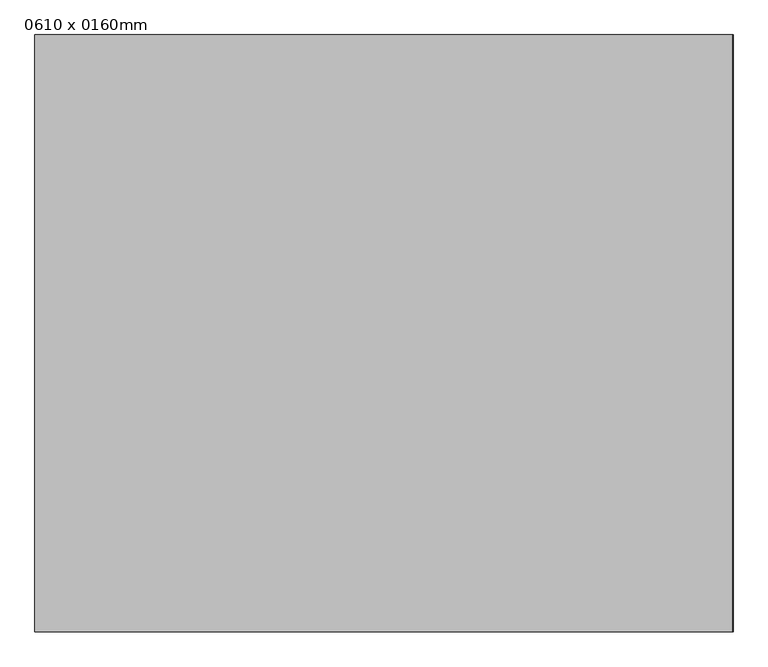
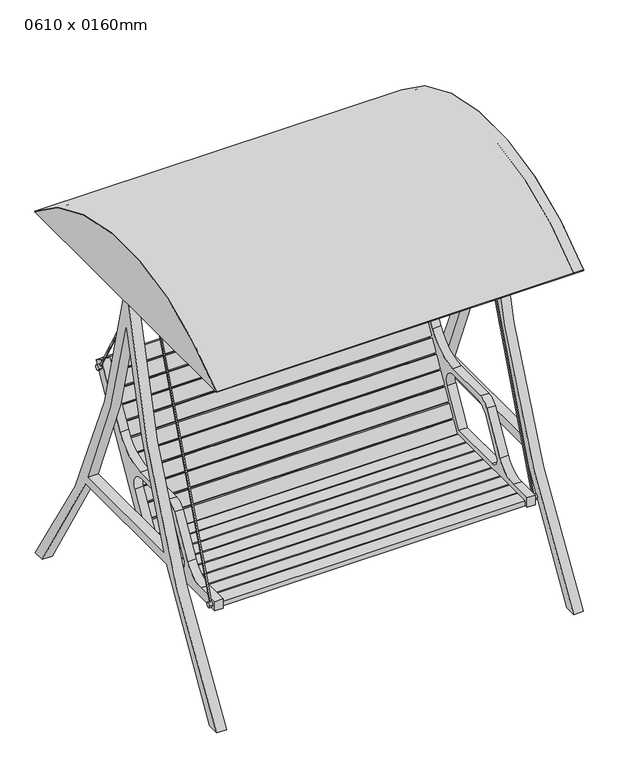
"""IFC4 building model written with IfcOpenShell, lengths in millimetres: furniture geometry, 0610 x 0160mm."""

from ifc_helpers import new_model, si_unit, point, frame, frame_2d, origin, place, context, project, spatial, polyline, circle_curve, trimmed, segment, composite_curve, outline, extrude, source, transform, mapped, element, save


def furniture_0610_x_0160mm_a8fad5e2(model_context):
    return source(origin(), model_context, "Body", "SweptSolid", [
        extrude(outline(composite_curve([segment(trimmed(circle_curve(frame_2d((4189.9023331, 1950.2809332)), 3303.1244251), [point((933.45, 1396.9734505))], [point((1524.0, 0.0))], True, "CARTESIAN"), True, "CONTINUOUS"), segment(polyline([(1524.0, 0.0), (1476.936255, 0.0)]), True, "CONTINUOUS"), segment(trimmed(circle_curve(frame_2d((4189.9023331, 1950.2809332)), 3341.2244251), [point((1476.936255, 0.0))], [point((1186.3373595, 486.5944542))], False, "CARTESIAN"), True, "CONTINUOUS"), segment(polyline([(1186.3373595, 486.5944542), (642.4626405, 486.5944542)]), True, "CONTINUOUS"), segment(trimmed(circle_curve(frame_2d((-2361.1023331, 1950.2809332)), 3341.2244251), [point((642.4626405, 486.5944542))], [point((351.863745, 0.0))], False, "CARTESIAN"), True, "CONTINUOUS"), segment(polyline([(351.863745, 0.0), (304.8, 0.0)]), True, "CONTINUOUS"), segment(trimmed(circle_curve(frame_2d((-2361.1023331, 1950.2809332)), 3303.1244251), [point((304.8, 0.0))], [point((895.35, 1396.9734505))], True, "CARTESIAN"), True, "CONTINUOUS"), segment(polyline([(895.35, 1396.9734505), (895.35, 1524.0), (914.4, 1524.0), (933.45, 1524.0), (933.45, 1396.9734505)]), True, "CONTINUOUS")], self_intersect=False), holes=[composite_curve([segment(polyline([(660.7321842, 524.6944542), (1168.0678158, 524.6944542)]), True, "CONTINUOUS"), segment(trimmed(circle_curve(frame_2d((4189.9023331, 1950.2809332)), 3341.2244251), [point((1168.0678158, 524.6944542))], [point((914.4, 1290.8378915))], False, "CARTESIAN"), True, "CONTINUOUS"), segment(trimmed(circle_curve(frame_2d((-2361.1023331, 1950.2809332)), 3341.2244251), [point((914.4, 1290.8378915))], [point((660.7321842, 524.6944542))], False, "CARTESIAN"), True, "CONTINUOUS")], self_intersect=False)]), frame((-272.362745, 0.0, 0.0), z_axis=(1.0, 0.0, 0.0), x_axis=(0.0, 1.0, 0.0)), (0.0, 0.0, 1.0), 38.1),
        extrude(outline(composite_curve([segment(trimmed(circle_curve(frame_2d((4189.9023331, 1950.2809332)), 3303.1244251), [point((933.45, 1396.9734505))], [point((1524.0, 0.0))], True, "CARTESIAN"), True, "CONTINUOUS"), segment(polyline([(1524.0, 0.0), (1476.936255, 0.0)]), True, "CONTINUOUS"), segment(trimmed(circle_curve(frame_2d((4189.9023331, 1950.2809332)), 3341.2244251), [point((1476.936255, 0.0))], [point((1186.3373595, 486.5944542))], False, "CARTESIAN"), True, "CONTINUOUS"), segment(polyline([(1186.3373595, 486.5944542), (642.4626405, 486.5944542)]), True, "CONTINUOUS"), segment(trimmed(circle_curve(frame_2d((-2361.1023331, 1950.2809332)), 3341.2244251), [point((642.4626405, 486.5944542))], [point((351.863745, 0.0))], False, "CARTESIAN"), True, "CONTINUOUS"), segment(polyline([(351.863745, 0.0), (304.8, 0.0)]), True, "CONTINUOUS"), segment(trimmed(circle_curve(frame_2d((-2361.1023331, 1950.2809332)), 3303.1244251), [point((304.8, 0.0))], [point((895.35, 1396.9734505))], True, "CARTESIAN"), True, "CONTINUOUS"), segment(polyline([(895.35, 1396.9734505), (895.35, 1524.0), (914.4, 1524.0), (933.45, 1524.0), (933.45, 1396.9734505)]), True, "CONTINUOUS")], self_intersect=False), holes=[composite_curve([segment(polyline([(660.7321842, 524.6944542), (1168.0678158, 524.6944542)]), True, "CONTINUOUS"), segment(trimmed(circle_curve(frame_2d((4189.9023331, 1950.2809332)), 3341.2244251), [point((1168.0678158, 524.6944542))], [point((914.4, 1290.8378915))], False, "CARTESIAN"), True, "CONTINUOUS"), segment(trimmed(circle_curve(frame_2d((-2361.1023331, 1950.2809332)), 3341.2244251), [point((914.4, 1290.8378915))], [point((660.7321842, 524.6944542))], False, "CARTESIAN"), True, "CONTINUOUS")], self_intersect=False)]), frame((1111.937255, 0.0, 0.0), z_axis=(1.0, 0.0, 0.0), x_axis=(0.0, 1.0, 0.0)), (0.0, 0.0, 1.0), 38.1),
        extrude(outline(polyline([(1111.937255, 933.45), (1111.937255, 895.35), (-234.262745, 895.35), (-234.262745, 933.45), (1111.937255, 933.45)])), frame((0.0, 0.0, 1484.1023899), z_axis=(0.0, 0.0, 1.0), x_axis=(1.0, 0.0, 0.0)), (0.0, 0.0, 1.0), 39.8976101),
        extrude(outline(composite_curve([segment(trimmed(circle_curve(frame_2d((914.4, 699.3747703)), 926.421113), [point((304.8, 1396.9734505))], [point((1524.0, 1396.9734505))], False, "CARTESIAN"), True, "CONTINUOUS"), segment(polyline([(1524.0, 1396.9734505), (304.8, 1396.9734505)]), True, "CONTINUOUS")], self_intersect=False), holes=[composite_curve([segment(polyline([(376.708681, 1422.3734505), (1452.091319, 1422.3734505)]), True, "CONTINUOUS"), segment(trimmed(circle_curve(frame_2d((914.4, 699.3747703)), 901.021113), [point((1452.091319, 1422.3734505))], [point((376.708681, 1422.3734505))], True, "CARTESIAN"), True, "CONTINUOUS")], self_intersect=False)]), frame((-272.362745, 0.0, 0.0), z_axis=(1.0, 0.0, 0.0), x_axis=(0.0, 1.0, 0.0)), (0.0, 0.0, 1.0), 38.1),
        extrude(outline(composite_curve([segment(trimmed(circle_curve(frame_2d((914.4, 699.3747703)), 926.421113), [point((304.8, 1396.9734505))], [point((1524.0, 1396.9734505))], False, "CARTESIAN"), True, "CONTINUOUS"), segment(polyline([(1524.0, 1396.9734505), (304.8, 1396.9734505)]), True, "CONTINUOUS")], self_intersect=False), holes=[composite_curve([segment(polyline([(376.708681, 1422.3734505), (1452.091319, 1422.3734505)]), True, "CONTINUOUS"), segment(trimmed(circle_curve(frame_2d((914.4, 699.3747703)), 901.021113), [point((1452.091319, 1422.3734505))], [point((376.708681, 1422.3734505))], True, "CARTESIAN"), True, "CONTINUOUS")], self_intersect=False)]), frame((1111.937255, 0.0, 0.0), z_axis=(1.0, 0.0, 0.0), x_axis=(0.0, 1.0, 0.0)), (0.0, 0.0, 1.0), 38.1),
        extrude(outline(composite_curve([segment(trimmed(circle_curve(frame_2d((914.4, 699.3747703)), 926.421113), [point((304.8, 1396.9734505))], [point((1524.0, 1396.9734505))], False, "CARTESIAN"), True, "CONTINUOUS"), segment(polyline([(1524.0, 1396.9734505), (304.8, 1396.9734505)]), True, "CONTINUOUS")], self_intersect=False)), frame((-273.952745, 0.0, 0.0), z_axis=(1.0, 0.0, 0.0), x_axis=(0.0, 1.0, 0.0)), (0.0, 0.0, 1.0), 1.59),
        extrude(outline(composite_curve([segment(trimmed(circle_curve(frame_2d((914.4, 699.3747703)), 926.421113), [point((304.8, 1396.9734505))], [point((1524.0, 1396.9734505))], False, "CARTESIAN"), True, "CONTINUOUS"), segment(polyline([(1524.0, 1396.9734505), (304.8, 1396.9734505)]), True, "CONTINUOUS")], self_intersect=False)), frame((1150.037255, 0.0, 0.0), z_axis=(1.0, 0.0, 0.0), x_axis=(0.0, 1.0, 0.0)), (0.0, 0.0, 1.0), 1.59),
        extrude(outline(composite_curve([segment(trimmed(circle_curve(frame_2d((914.4, 699.3747703)), 926.421113), [point((1524.0, 1396.9734505))], [point((304.8, 1396.9734505))], True, "CARTESIAN"), True, "CONTINUOUS"), segment(polyline([(304.8, 1396.9734505), (304.8, 1399.0836139)]), True, "CONTINUOUS"), segment(trimmed(circle_curve(frame_2d((914.4, 699.3747703)), 928.011113), [point((304.8, 1399.0836139))], [point((1524.0, 1399.0836139))], False, "CARTESIAN"), True, "CONTINUOUS"), segment(polyline([(1524.0, 1399.0836139), (1524.0, 1396.9734505)]), True, "CONTINUOUS")], self_intersect=False)), frame((-273.952745, 0.0, 0.0), z_axis=(1.0, 0.0, 0.0), x_axis=(0.0, 1.0, 0.0)), (0.0, 0.0, 1.0), 1423.99),
        extrude(outline(composite_curve([segment(trimmed(circle_curve(frame_2d((563.6419667, 511.4)), 105.0), [point((563.6419667, 406.4))], [point((654.5746341, 458.9))], True, "CARTESIAN"), True, "CONTINUOUS"), segment(polyline([(654.5746341, 458.9), (741.8122598, 610.0)]), True, "CONTINUOUS"), segment(trimmed(circle_curve(frame_2d((785.11353, 585.0)), 50.0), [point((741.8122598, 610.0))], [point((785.11353, 635.0))], False, "CARTESIAN"), True, "CONTINUOUS"), segment(polyline([(785.11353, 635.0), (968.6699734, 635.0)]), True, "CONTINUOUS"), segment(trimmed(circle_curve(frame_2d((968.6699734, 795.0)), 160.0), [point((968.6699734, 635.0))], [point((1107.2340381, 715.0))], True, "CARTESIAN"), True, "CONTINUOUS"), segment(polyline([(1107.2340381, 715.0), (1233.863745, 934.3290861), (1266.8593129, 915.2790861), (951.0607902, 368.3), (471.863745, 368.3), (471.863745, 406.4), (563.6419667, 406.4)]), True, "CONTINUOUS")], self_intersect=False), holes=[composite_curve([segment(trimmed(circle_curve(frame_2d((807.1413638, 546.8466726)), 62.7533274), [point((807.1413638, 609.6))], [point((752.7953881, 578.2233363))], True, "CARTESIAN"), True, "CONTINUOUS"), segment(polyline([(752.7953881, 578.2233363), (679.5739008, 451.4)]), True, "CONTINUOUS"), segment(trimmed(circle_curve(frame_2d((705.5546629, 436.4)), 30.0), [point((679.5739008, 451.4))], [point((705.5546629, 406.4))], True, "CARTESIAN"), True, "CONTINUOUS"), segment(polyline([(705.5546629, 406.4), (929.063745, 406.4), (1007.4101765, 542.1)]), True, "CONTINUOUS"), segment(trimmed(circle_curve(frame_2d((968.4390333, 564.6)), 45.0), [point((1007.4101765, 542.1))], [point((968.4390333, 609.6))], True, "CARTESIAN"), True, "CONTINUOUS"), segment(polyline([(968.4390333, 609.6), (807.1413638, 609.6)]), True, "CONTINUOUS")], self_intersect=False)]), frame((-184.03019, 0.0, 0.0), z_axis=(1.0, 0.0, 0.0), x_axis=(0.0, 1.0, 0.0)), (0.0, 0.0, 1.0), 32.5713093),
        extrude(outline(composite_curve([segment(trimmed(circle_curve(frame_2d((563.6419667, 511.4)), 105.0), [point((563.6419667, 406.4))], [point((654.5746341, 458.9))], True, "CARTESIAN"), True, "CONTINUOUS"), segment(polyline([(654.5746341, 458.9), (741.8122598, 610.0)]), True, "CONTINUOUS"), segment(trimmed(circle_curve(frame_2d((785.11353, 585.0)), 50.0), [point((741.8122598, 610.0))], [point((785.11353, 635.0))], False, "CARTESIAN"), True, "CONTINUOUS"), segment(polyline([(785.11353, 635.0), (968.6699734, 635.0)]), True, "CONTINUOUS"), segment(trimmed(circle_curve(frame_2d((968.6699734, 795.0)), 160.0), [point((968.6699734, 635.0))], [point((1107.2340381, 715.0))], True, "CARTESIAN"), True, "CONTINUOUS"), segment(polyline([(1107.2340381, 715.0), (1233.863745, 934.3290861), (1266.8593129, 915.2790861), (951.0607902, 368.3), (471.863745, 368.3), (471.863745, 406.4), (563.6419667, 406.4)]), True, "CONTINUOUS")], self_intersect=False), holes=[composite_curve([segment(trimmed(circle_curve(frame_2d((807.1413638, 546.8466726)), 62.7533274), [point((807.1413638, 609.6))], [point((752.7953881, 578.2233363))], True, "CARTESIAN"), True, "CONTINUOUS"), segment(polyline([(752.7953881, 578.2233363), (679.5739008, 451.4)]), True, "CONTINUOUS"), segment(trimmed(circle_curve(frame_2d((705.5546629, 436.4)), 30.0), [point((679.5739008, 451.4))], [point((705.5546629, 406.4))], True, "CARTESIAN"), True, "CONTINUOUS"), segment(polyline([(705.5546629, 406.4), (929.063745, 406.4), (1007.4101765, 542.1)]), True, "CONTINUOUS"), segment(trimmed(circle_curve(frame_2d((968.4390333, 564.6)), 45.0), [point((1007.4101765, 542.1))], [point((968.4390333, 609.6))], True, "CARTESIAN"), True, "CONTINUOUS"), segment(polyline([(968.4390333, 609.6), (807.1413638, 609.6)]), True, "CONTINUOUS")], self_intersect=False)]), frame((1027.5433908, 0.0, 0.0), z_axis=(1.0, 0.0, 0.0), x_axis=(0.0, 1.0, 0.0)), (0.0, 0.0, 1.0), 32.5713093),
        extrude(outline(polyline([(0.0, -19.0500001), (0.0, 0.0), (1179.0022715, 0.0), (1179.0022715, -19.0500001), (0.0, -19.0500001)])), frame((1027.5433908, 1224.9615289, 880.8099956), z_axis=(0.0, 0.5000000000000067, 0.8660254037844349), x_axis=(-1.0, 0.0, 0.0)), (0.0, 0.0, 1.0), 50.8),
        extrude(outline(polyline([(0.0, -19.0500001), (0.0, 0.0), (1179.0022715, 0.0), (1179.0022715, -19.0500001), (0.0, -19.0500001)])), frame((1027.5433908, 1196.3865289, 831.3166438), z_axis=(0.0, 0.5000000000000067, 0.8660254037844349), x_axis=(-1.0, 0.0, 0.0)), (0.0, 0.0, 1.0), 50.8),
        extrude(outline(polyline([(0.0, -19.0500001), (0.0, 0.0), (1179.0022715, 0.0), (1179.0022715, -19.0500001), (0.0, -19.0500001)])), frame((1027.5433908, 1167.8115289, 781.823292), z_axis=(0.0, 0.5000000000000067, 0.8660254037844349), x_axis=(-1.0, 0.0, 0.0)), (0.0, 0.0, 1.0), 50.8),
        extrude(outline(polyline([(0.0, -19.0500001), (0.0, 0.0), (1179.0022715, 0.0), (1179.0022715, -19.0500001), (0.0, -19.0500001)])), frame((1027.5433908, 1139.2365289, 732.3299402), z_axis=(0.0, 0.5000000000000067, 0.8660254037844349), x_axis=(-1.0, 0.0, 0.0)), (0.0, 0.0, 1.0), 50.8),
        extrude(outline(polyline([(0.0, -19.0500001), (0.0, 0.0), (1179.0022715, 0.0), (1179.0022715, -19.0500001), (0.0, -19.0500001)])), frame((1027.5433908, 1110.6615289, 682.8365883), z_axis=(0.0, 0.5000000000000067, 0.8660254037844349), x_axis=(-1.0, 0.0, 0.0)), (0.0, 0.0, 1.0), 50.8),
        extrude(outline(polyline([(0.0, -19.0500001), (0.0, 0.0), (1179.0022715, 0.0), (1179.0022715, -19.0500001), (0.0, -19.0500001)])), frame((1027.5433908, 1082.0865289, 633.3432365), z_axis=(0.0, 0.5000000000000067, 0.8660254037844349), x_axis=(-1.0, 0.0, 0.0)), (0.0, 0.0, 1.0), 50.8),
        extrude(outline(polyline([(0.0, -19.0500001), (0.0, 0.0), (1179.0022715, 0.0), (1179.0022715, -19.0500001), (0.0, -19.0500001)])), frame((1027.5433908, 1053.5115289, 583.8498847), z_axis=(0.0, 0.5000000000000067, 0.8660254037844349), x_axis=(-1.0, 0.0, 0.0)), (0.0, 0.0, 1.0), 50.8),
        extrude(outline(polyline([(0.0, -19.0500001), (0.0, 0.0), (1179.0022715, 0.0), (1179.0022715, -19.0500001), (0.0, -19.0500001)])), frame((1027.5433908, 1024.9365289, 534.3565329), z_axis=(0.0, 0.5000000000000067, 0.8660254037844349), x_axis=(-1.0, 0.0, 0.0)), (0.0, 0.0, 1.0), 50.8),
        extrude(outline(polyline([(0.0, -19.0500001), (0.0, 0.0), (1179.0022715, 0.0), (1179.0022715, -19.0500001), (0.0, -19.0500001)])), frame((1027.5433908, 996.3615289, 484.863181), z_axis=(0.0, 0.5000000000000067, 0.8660254037844349), x_axis=(-1.0, 0.0, 0.0)), (0.0, 0.0, 1.0), 50.8),
        extrude(outline(polyline([(0.0, -19.0500001), (0.0, 0.0), (1179.0022715, 0.0), (1179.0022715, -19.0500001), (0.0, -19.0500001)])), frame((1027.5433908, 967.7865289, 435.3698292), z_axis=(0.0, 0.5000000000000067, 0.8660254037844349), x_axis=(-1.0, 0.0, 0.0)), (0.0, 0.0, 1.0), 50.8),
        extrude(outline(polyline([(0.0, -19.0500001), (0.0, 0.0), (1179.0022715, 0.0), (1179.0022715, -19.0500001), (0.0, -19.0500001)])), frame((1027.5433908, 939.2115289, 385.8764774), z_axis=(0.0, 0.5000000000000067, 0.8660254037844349), x_axis=(-1.0, 0.0, 0.0)), (0.0, 0.0, 1.0), 50.8),
        extrude(outline(polyline([(1027.5433908, 933.8211), (1027.5433908, 883.0211), (-151.4588807, 883.0211), (-151.4588807, 933.8211), (1027.5433908, 933.8211)])), frame((0.0, 0.0, 368.3), z_axis=(0.0, 0.0, 1.0), x_axis=(1.0, 0.0, 0.0)), (0.0, 0.0, 1.0), 19.05),
        extrude(outline(polyline([(1027.5433908, 876.6711), (1027.5433908, 825.8711), (-151.4588807, 825.8711), (-151.4588807, 876.6711), (1027.5433908, 876.6711)])), frame((0.0, 0.0, 368.3), z_axis=(0.0, 0.0, 1.0), x_axis=(1.0, 0.0, 0.0)), (0.0, 0.0, 1.0), 19.05),
        extrude(outline(polyline([(1027.5433908, 819.5211), (1027.5433908, 768.7211), (-151.4588807, 768.7211), (-151.4588807, 819.5211), (1027.5433908, 819.5211)])), frame((0.0, 0.0, 368.3), z_axis=(0.0, 0.0, 1.0), x_axis=(1.0, 0.0, 0.0)), (0.0, 0.0, 1.0), 19.05),
        extrude(outline(polyline([(1027.5433908, 762.3711), (1027.5433908, 711.5711), (-151.4588807, 711.5711), (-151.4588807, 762.3711), (1027.5433908, 762.3711)])), frame((0.0, 0.0, 368.3), z_axis=(0.0, 0.0, 1.0), x_axis=(1.0, 0.0, 0.0)), (0.0, 0.0, 1.0), 19.05),
        extrude(outline(polyline([(1027.5433908, 705.2211), (1027.5433908, 654.4211), (-151.4588807, 654.4211), (-151.4588807, 705.2211), (1027.5433908, 705.2211)])), frame((0.0, 0.0, 368.3), z_axis=(0.0, 0.0, 1.0), x_axis=(1.0, 0.0, 0.0)), (0.0, 0.0, 1.0), 19.05),
        extrude(outline(polyline([(1027.5433908, 648.0711), (1027.5433908, 597.2711), (-151.4588807, 597.2711), (-151.4588807, 648.0711), (1027.5433908, 648.0711)])), frame((0.0, 0.0, 368.3), z_axis=(0.0, 0.0, 1.0), x_axis=(1.0, 0.0, 0.0)), (0.0, 0.0, 1.0), 19.05),
        extrude(outline(polyline([(1027.5433908, 590.9211), (1027.5433908, 540.1211), (-151.4588807, 540.1211), (-151.4588807, 590.9211), (1027.5433908, 590.9211)])), frame((0.0, 0.0, 368.3), z_axis=(0.0, 0.0, 1.0), x_axis=(1.0, 0.0, 0.0)), (0.0, 0.0, 1.0), 19.05),
        extrude(outline(polyline([(1027.5433908, 533.7711), (1027.5433908, 482.9711), (-151.4588807, 482.9711), (-151.4588807, 533.7711), (1027.5433908, 533.7711)])), frame((0.0, 0.0, 368.3), z_axis=(0.0, 0.0, 1.0), x_axis=(1.0, 0.0, 0.0)), (0.0, 0.0, 1.0), 19.05),
        extrude(outline(polyline([(914.4, 1484.1023899), (1241.1891484, 905.4891111), (1236.3748088, 902.7700689), (911.842017, 1477.3882398), (494.9813942, 383.2195737), (489.4362629, 385.3321793), (908.05, 1484.1023899), (914.4, 1484.1023899)])), frame((-188.7825876, 0.0, 0.0), z_axis=(1.0, 0.0, 0.0), x_axis=(0.0, 1.0, 0.0)), (0.0, 0.0, 1.0), 4.7523976),
        extrude(outline(composite_curve([segment(trimmed(circle_curve(frame_2d((1238.7819786, 904.12959)), 10.0), [point((1228.7819786, 904.12959))], [point((1248.7819786, 904.12959))], False, "CARTESIAN"), True, "CONTINUOUS"), segment(trimmed(circle_curve(frame_2d((1238.7819786, 904.12959)), 10.0), [point((1248.7819786, 904.12959))], [point((1228.7819786, 904.12959))], False, "CARTESIAN"), True, "CONTINUOUS")], self_intersect=False)), frame((-196.8218142, 0.0, 0.0), z_axis=(1.0, 0.0, 0.0), x_axis=(0.0, 1.0, 0.0)), (0.0, 0.0, 1.0), 12.7916242),
        extrude(outline(composite_curve([segment(trimmed(circle_curve(frame_2d((492.2088285, 384.2758765)), 10.0), [point((482.2088285, 384.2758765))], [point((502.2088285, 384.2758765))], False, "CARTESIAN"), True, "CONTINUOUS"), segment(trimmed(circle_curve(frame_2d((492.2088285, 384.2758765)), 10.0), [point((502.2088285, 384.2758765))], [point((482.2088285, 384.2758765))], False, "CARTESIAN"), True, "CONTINUOUS")], self_intersect=False)), frame((-196.8218142, 0.0, 0.0), z_axis=(1.0, 0.0, 0.0), x_axis=(0.0, 1.0, 0.0)), (0.0, 0.0, 1.0), 12.7916242),
        extrude(outline(polyline([(914.4, 1484.1023899), (1241.1891484, 905.4891111), (1236.3748088, 902.7700689), (911.842017, 1477.3882398), (494.9813942, 383.2195737), (489.4362629, 385.3321793), (908.05, 1484.1023899), (914.4, 1484.1023899)])), frame((1061.7047, 0.0, 0.0), z_axis=(1.0, 0.0, 0.0), x_axis=(0.0, 1.0, 0.0)), (0.0, 0.0, 1.0), 4.7523976),
        extrude(outline(composite_curve([segment(trimmed(circle_curve(frame_2d((1238.7819786, 904.12959)), 10.0), [point((1228.7819786, 904.12959))], [point((1248.7819786, 904.12959))], False, "CARTESIAN"), True, "CONTINUOUS"), segment(trimmed(circle_curve(frame_2d((1238.7819786, 904.12959)), 10.0), [point((1248.7819786, 904.12959))], [point((1228.7819786, 904.12959))], False, "CARTESIAN"), True, "CONTINUOUS")], self_intersect=False)), frame((1061.7047, 0.0, 0.0), z_axis=(1.0, 0.0, 0.0), x_axis=(0.0, 1.0, 0.0)), (0.0, 0.0, 1.0), 12.7916242),
        extrude(outline(composite_curve([segment(trimmed(circle_curve(frame_2d((492.2088285, 384.2758765)), 10.0), [point((482.2088285, 384.2758765))], [point((502.2088285, 384.2758765))], False, "CARTESIAN"), True, "CONTINUOUS"), segment(trimmed(circle_curve(frame_2d((492.2088285, 384.2758765)), 10.0), [point((502.2088285, 384.2758765))], [point((482.2088285, 384.2758765))], False, "CARTESIAN"), True, "CONTINUOUS")], self_intersect=False)), frame((1061.7047, 0.0, 0.0), z_axis=(1.0, 0.0, 0.0), x_axis=(0.0, 1.0, 0.0)), (0.0, 0.0, 1.0), 12.7916242),
    ])


if __name__ == "__main__":
    model = new_model("IFC4")
    model_context = context("Model", 3, world=origin())
    ifc_project = project(units=[si_unit("LENGTHUNIT", "METRE", prefix="MILLI")], contexts=[model_context])
    site = spatial("IfcSite", under=ifc_project)
    building = spatial("IfcBuilding", under=site)
    placement = place(None, origin())
    furniture_0610_x_0160mm_shape = furniture_0610_x_0160mm_a8fad5e2(model_context)
    element("IfcFurniture", 1, ObjectType="0610 x 0160mm", at=placement, inside=building, context=model_context, shape_type="MappedRepresentation", body=[
        mapped(furniture_0610_x_0160mm_shape, transform((0.0, 0.0, 0.0), x_axis=(1.0, 0.0, 0.0), y_axis=(0.0, 1.0, 0.0), z_axis=(0.0, 0.0, 1.0))),
    ])
    save(model, "model.ifc")

# Revit data of these elements
# Type "0610 x 0160mm"
#   Height = 2' - 6"
#   Length = 2' - 0.01575"
#   Width = 2' - 0.01575"
#   Base Material = Wood - Birch
#   Top Material = Laminate - Ivory, Matte
#   Default Elevation = 0
# Element 1 (IfcFurniture, "0610 x 0160mm")
#   Materials on its faces: "wood finish", "steel", "Laminate - Ivory, Matte", "fabric"
# Materials
#   "Wood - Birch": colour RGB 230 196 162, transparency 0
#   "Laminate - Ivory, Matte": colour RGB 247 247 239, transparency 0
#   "wood finish": class "Generic", colour RGB 120 120 120, transparency 0, Cost = 0
#   "steel": class "Generic", colour RGB 120 120 120, transparency 0, Cost = 0
#   "fabric": class "Generic", colour RGB 120 120 120, transparency 0, Cost = 0
